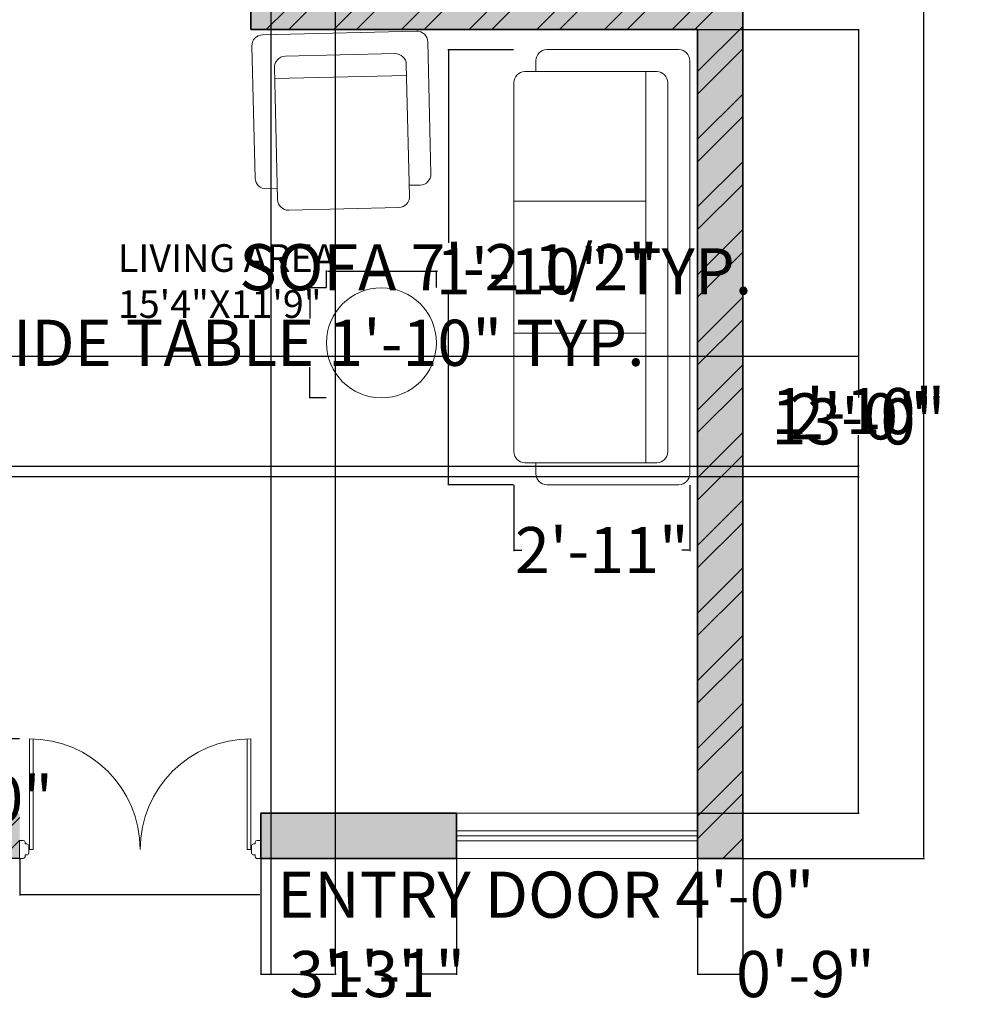
# Model space of a CAD drawing. Units: inches. Extents: x 1086 to 1540, y 3343 to 3848.
# Tile 2 of 8: x 1327 to 1515, y 3351 to 3547. Entities that reach past the tile are written whole.
import ezdxf

# ---------------------------------------------------------------- set-up
doc = ezdxf.new("R2010")
doc.units = ezdxf.units.IN
for name, color, linetype, lineweight in [('00 FURNITURE', 15, 'Continuous', 15), ('A-ANNO-DIMS', 2, 'Continuous', 13), ('A-AREA-IDEN', 7, 'Continuous', 18), ('A-DOOR', 4, 'Continuous', 20), ('A-WALL-PATT', 252, 'Continuous', 9), ('WALL', 7, 'Continuous', 35), ('WINDOW', 160, 'Continuous', 15)]:
    doc.layers.add(name, color=color, linetype=linetype, lineweight=lineweight)
doc.styles.get("Standard").update_dxf_attribs({"font": 'arial.ttf'})
doc.dimstyles.get("Standard").update_dxf_attribs({"dimtxt": 9.18, "dimasz": 0.18, "dimexe": 0.18, "dimexo": 0.0625, "dimgap": 0.09, "dimtad": 0, "dimtih": 1, "dimtoh": 1, "dimdec": 1, "dimzin": 0, "dimdsep": 46, "dimlunit": 3, "dimtxsty": 'Standard', "dimcen": 0.09, "dimadec": 0, "dimazin": 0, "dimtfac": 1, "dimtdec": 1, "dimtofl": 0, "dimtmove": 0, "dimatfit": 3, "dimfxl": 1, "dimtolj": 1, "dimtzin": 0, "dimarcsym": 0})

# ---------------------------------------------------------------- blocks, each defined once
blk = doc.blocks.new('PUJA')
at = {"layer": '00 FURNITURE'}
for p, q in [((-1941.8, -16091.75), (-1938.89, -16091.75)), ((-1941.8, -16092.33), (-1941.8, -16091.75)), ((-1938.89, -16091.75), (-1938.89, -16092.33)), ((-1940.35, -16093.35), (-1958.14, -16093.35)), ((-1940.35, -16093.93), (-1958.13, -16093.93)), ((-1941.22, -16092.62), (-1941.51, -16092.62)), ((-1940.35, -16093.35), (-1940.35, -16093.93)), ((-1939.18, -16092.62), (-1939.47, -16092.62)), ((-1940.35, -16128.93), (-1958.14, -16128.93)), ((-1940.35, -16128.35), (-1958.13, -16128.35)), ((-1940.35, -16128.93), (-1940.35, -16128.35)), ((-1941.8, -16129.96), (-1941.8, -16130.54)), ((-1941.8, -16130.54), (-1938.89, -16130.54)), ((-1941.22, -16129.66), (-1941.51, -16129.66)), ((-1939.18, -16129.66), (-1939.47, -16129.66)), ((-1938.89, -16130.54), (-1938.89, -16129.96))]:
    blk.add_line(p, q, dxfattribs=at)
for points in [[(-1939.47, -16092.62), (-1939.47, -16092.91, -0.414214), (-1939.76, -16093.21), (-1940.93, -16093.21, -0.414214), (-1941.22, -16092.91), (-1941.22, -16092.62)], [(-1939.47, -16129.66), (-1939.47, -16129.37, 0.414214), (-1939.76, -16129.08), (-1940.93, -16129.08, 0.414214), (-1941.22, -16129.37), (-1941.22, -16129.66)]]:
    blk.add_lwpolyline(points, format="xyb", dxfattribs=at)
for centre, radius, start, end in [((-1941.51, -16092.33), 0.292, 180, 270), ((-1939.18, -16092.33), 0.292, 270, 0), ((-1940.35, -16093.35), 17.79, 180, 270), ((-1940.35, -16128.93), 17.79, 90, 180), ((-1941.51, -16129.96), 0.292, 90, 180), ((-1939.18, -16129.96), 0.292, 0, 90)]:
    blk.add_arc(centre, radius, start, end, dxfattribs=at)
blk = doc.blocks.new('sofa 6')
for p, q in [((-1044.4, 890), (1044.4, 890)), ((-1100, 166.9), (-1100, 834.3)), ((1100, 834.3), (1100, 166.9)), ((-933.1, 778.7), (933.1, 778.7)), ((-988.8, 55.6), (-988.8, 723.1)), ((988.8, 723.1), (988.8, 55.6)), ((-988.8, 667.5), (988.8, 667.5)), ((-333.8, 667.5), (-333.8, 0)), ((333.7, 667.5), (333.7, 0)), ((-988.8, 111.2), (-1044.4, 111.2)), ((1044.4, 111.2), (988.8, 111.2)), ((933.1, 0), (-933.1, 0))]:
    blk.add_line(p, q)
for centre, start, end in [((-1044.4, 834.3), 90, 180), ((1044.4, 834.3), 0, 90), ((-933.1, 723.1), 90, 180), ((933.1, 723.1), 0, 90), ((-1044.4, 166.9), 180, 270), ((1044.4, 166.9), 270, 0), ((-933.1, 55.6), 180, 270), ((933.1, 55.6), 270, 0)]:
    blk.add_arc(centre, 55.6, start, end)
blk = doc.blocks.new('chair')
at = {"layer": '00 FURNITURE'}
for p, q in [((1375.85, 3529.75), (1402.12, 3529.75)), ((1373.66, 3525.37), (1373.66, 3527.56)), ((1404.31, 3527.56), (1404.31, 3496.9)), ((1371.47, 3525.37), (1397.74, 3525.37)), ((1395.55, 3525.37), (1395.55, 3499.09)), ((1369.28, 3501.28), (1369.28, 3523.18)), ((1399.93, 3523.18), (1399.93, 3501.28)), ((1397.74, 3499.09), (1371.47, 3499.09)), ((1373.66, 3496.9), (1373.66, 3499.09)), ((1402.12, 3494.71), (1375.85, 3494.71))]:
    blk.add_line(p, q, dxfattribs=at)
for centre, start, end in [((1375.85, 3527.56), 90, 180), ((1402.12, 3527.56), 0, 90), ((1371.47, 3523.18), 90, 180), ((1397.74, 3523.18), 0, 90), ((1371.47, 3501.28), 180, 270), ((1397.74, 3501.28), 270, 0), ((1375.85, 3496.9), 180, 270), ((1402.12, 3496.9), 270, 0)]:
    blk.add_arc(centre, 2.19, start, end, dxfattribs=at)
blk = doc.blocks.new('*D13')
at = {"layer": 'A-ANNO-DIMS', "color": 0, "lineweight": -2, "transparency": 16777216}
for p, q in [((1470.8, 3811.57), (1506.93, 3811.57)), ((1506.75, 3811.39), (1506.75, 3600.35)), ((1506.75, 3379.75), (1506.75, 3590.79)), ((1470.8, 3379.57), (1506.93, 3379.57))]:
    blk.add_line(p, q, dxfattribs=at)
at = {"layer": 'A-ANNO-DIMS', "color": 0, "transparency": 16777216}
for points in [[(1506.72, 3811.39), (1506.78, 3811.39), (1506.75, 3811.57)], [(1506.72, 3379.75), (1506.78, 3379.75), (1506.75, 3379.57)]]:
    blk.add_solid(points, dxfattribs=at)
at = {"layer": 'Defpoints', "color": 0, "transparency": 16777216}
for p in [(1470.74, 3811.57), (1470.74, 3379.57), (1506.75, 3379.57)]:
    blk.add_point(p, dxfattribs=at)
at = {"layer": 'A-ANNO-DIMS', "color": 0, "transparency": 16777216, "insert": (1506.75, 3595.57), "char_height": 9.18, "attachment_point": 5}
blk.add_mtext("\\A1;36'", dxfattribs=at)
blk = doc.blocks.new('WIN-GLAZING-48IN')
for p, q in [((48, 1), (0, 1)), ((48, 0), (0, 0)), ((48, -1), (0, -1))]:
    blk.add_line(p, q)
blk = doc.blocks.new('TABLE-ROUND-SIDE')
blk.add_circle((0, 0), 10.95)
blk = doc.blocks.new('*D29')
at = {"layer": 'A-ANNO-DIMS', "color": 0, "lineweight": -2, "transparency": 16777216}
for p, q in [((1387.77, 3493.16), (1384.37, 3493.16)), ((1384.55, 3492.98), (1384.55, 3487.04)), ((1384.55, 3471.44), (1384.55, 3477.37)), ((1387.77, 3471.26), (1384.37, 3471.26))]:
    blk.add_line(p, q, dxfattribs=at)
at = {"layer": 'A-ANNO-DIMS', "color": 0, "transparency": 16777216}
for points in [[(1384.52, 3492.98), (1384.58, 3492.98), (1384.55, 3493.16)], [(1384.52, 3471.44), (1384.58, 3471.44), (1384.55, 3471.26)]]:
    blk.add_solid(points, dxfattribs=at)
at = {"layer": 'Defpoints', "color": 0, "transparency": 16777216}
for p in [(1384.55, 3493.16), (1387.83, 3493.16), (1387.83, 3471.26)]:
    blk.add_point(p, dxfattribs=at)
at = {"layer": 'A-ANNO-DIMS', "color": 0, "transparency": 16777216, "insert": (1384.55, 3482.21), "char_height": 9.18, "attachment_point": 5}
blk.add_mtext('\\A1;SIDE TABLE 1\'-10" TYP.', dxfattribs=at)
blk = doc.blocks.new('*D30')
at = {"layer": 'A-ANNO-DIMS', "color": 0, "lineweight": -2, "transparency": 16777216}
for p, q in [((1387.83, 3493.22), (1387.83, 3496.62)), ((1388.01, 3496.44), (1409.55, 3496.44)), ((1409.73, 3493.22), (1409.73, 3496.62)), ((1409.73, 3496.44), (1409.91, 3496.44))]:
    blk.add_line(p, q, dxfattribs=at)
at = {"layer": 'A-ANNO-DIMS', "color": 0, "transparency": 16777216}
for points in [[(1388.01, 3496.47), (1388.01, 3496.41), (1387.83, 3496.44)], [(1409.55, 3496.47), (1409.55, 3496.41), (1409.73, 3496.44)]]:
    blk.add_solid(points, dxfattribs=at)
at = {"layer": 'Defpoints', "color": 0, "transparency": 16777216}
for p in [(1409.73, 3496.44), (1387.83, 3493.16), (1409.73, 3493.16)]:
    blk.add_point(p, dxfattribs=at)
at = {"layer": 'A-ANNO-DIMS', "color": 0, "transparency": 16777216, "insert": (1441.11, 3496.44), "char_height": 9.18, "attachment_point": 5}
blk.add_mtext('\\A1;1\'-10" TYP.', dxfattribs=at)
blk = doc.blocks.new('*D43')
at = {"layer": 'A-ANNO-DIMS', "color": 0, "lineweight": -2, "transparency": 16777216}
for p, q in [((1326.74, 3379.51), (1326.74, 3372.19)), ((1374.74, 3379.51), (1374.74, 3372.19)), ((1326.92, 3372.37), (1374.56, 3372.37)), ((1374.74, 3372.37), (1374.92, 3372.37))]:
    blk.add_line(p, q, dxfattribs=at)
at = {"layer": 'A-ANNO-DIMS', "color": 0, "transparency": 16777216}
for points in [[(1326.92, 3372.4), (1326.92, 3372.34), (1326.74, 3372.37)], [(1374.56, 3372.4), (1374.56, 3372.34), (1374.74, 3372.37)]]:
    blk.add_solid(points, dxfattribs=at)
at = {"layer": 'Defpoints', "color": 0, "transparency": 16777216}
for p in [(1326.74, 3379.57), (1374.74, 3379.57), (1374.74, 3372.37)]:
    blk.add_point(p, dxfattribs=at)
at = {"layer": 'A-ANNO-DIMS', "color": 0, "transparency": 16777216, "insert": (1431.5, 3372.37), "char_height": 9.18, "attachment_point": 5}
blk.add_mtext('\\A1;ENTRY DOOR 4\'-0"', dxfattribs=at)
blk = doc.blocks.new('*D44')
at = {"layer": 'A-ANNO-DIMS', "color": 0, "lineweight": -2, "transparency": 16777216}
for p, q in [((1326.68, 3403.39), (1319.36, 3403.39)), ((1319.54, 3403.21), (1319.54, 3396.26)), ((1319.54, 3379.75), (1319.54, 3386.7)), ((1326.68, 3379.57), (1319.36, 3379.57))]:
    blk.add_line(p, q, dxfattribs=at)
at = {"layer": 'A-ANNO-DIMS', "color": 0, "transparency": 16777216}
for points in [[(1319.51, 3403.21), (1319.57, 3403.21), (1319.54, 3403.39)], [(1319.51, 3379.75), (1319.57, 3379.75), (1319.54, 3379.57)]]:
    blk.add_solid(points, dxfattribs=at)
at = {"layer": 'Defpoints', "color": 0, "transparency": 16777216}
for p in [(1326.74, 3403.39), (1319.54, 3379.57), (1326.74, 3379.57)]:
    blk.add_point(p, dxfattribs=at)
at = {"layer": 'A-ANNO-DIMS', "color": 0, "transparency": 16777216, "insert": (1319.54, 3391.48), "char_height": 9.18, "attachment_point": 5}
blk.add_mtext('\\A1;2\'-0"', dxfattribs=at)
blk = doc.blocks.new('*D45')
at = {"layer": 'A-ANNO-DIMS', "color": 0, "lineweight": -2, "transparency": 16777216}
for p, q in [((1425.08, 3540.55), (1411.97, 3540.55)), ((1412.15, 3540.37), (1412.15, 3502.09)), ((1412.15, 3454.12), (1412.15, 3492.41)), ((1425.08, 3453.94), (1411.97, 3453.94))]:
    blk.add_line(p, q, dxfattribs=at)
at = {"layer": 'A-ANNO-DIMS', "color": 0, "transparency": 16777216}
for points in [[(1412.12, 3540.37), (1412.18, 3540.37), (1412.15, 3540.55)], [(1412.12, 3454.12), (1412.18, 3454.12), (1412.15, 3453.94)]]:
    blk.add_solid(points, dxfattribs=at)
at = {"layer": 'Defpoints', "color": 0, "transparency": 16777216}
for p in [(1425.14, 3540.55), (1412.15, 3453.94), (1425.14, 3453.94)]:
    blk.add_point(p, dxfattribs=at)
at = {"layer": 'A-ANNO-DIMS', "color": 0, "transparency": 16777216, "insert": (1412.15, 3497.25), "char_height": 9.18, "attachment_point": 5}
blk.add_mtext('\\A1;SOFA 7\'-2 1/2"', dxfattribs=at)
blk = doc.blocks.new('*D46')
at = {"layer": 'A-ANNO-DIMS', "color": 0, "lineweight": -2, "transparency": 16777216}
for p, q in [((1425.14, 3453.88), (1425.14, 3440.77)), ((1460.18, 3453.88), (1460.18, 3440.77)), ((1425.32, 3440.95), (1426.72, 3440.95)), ((1460, 3440.95), (1458.59, 3440.95))]:
    blk.add_line(p, q, dxfattribs=at)
at = {"layer": 'A-ANNO-DIMS', "color": 0, "transparency": 16777216}
for points in [[(1425.32, 3440.98), (1425.32, 3440.92), (1425.14, 3440.95)], [(1460, 3440.98), (1460, 3440.92), (1460.18, 3440.95)]]:
    blk.add_solid(points, dxfattribs=at)
at = {"layer": 'Defpoints', "color": 0, "transparency": 16777216}
for p in [(1425.14, 3453.94), (1460.18, 3453.94), (1460.18, 3440.95)]:
    blk.add_point(p, dxfattribs=at)
at = {"layer": 'A-ANNO-DIMS', "color": 0, "transparency": 16777216, "insert": (1442.66, 3440.95), "char_height": 9.18, "attachment_point": 5}
blk.add_mtext('\\A1;2\'-11"', dxfattribs=at)
blk = doc.blocks.new('*D49')
at = {"layer": 'A-ANNO-DIMS', "color": 0, "lineweight": -2, "transparency": 16777216}
for p, q in [((1374.74, 3379.51), (1374.74, 3356.39)), ((1413.74, 3379.51), (1413.74, 3356.39)), ((1374.92, 3356.57), (1381.95, 3356.57)), ((1413.56, 3356.57), (1406.53, 3356.57))]:
    blk.add_line(p, q, dxfattribs=at)
at = {"layer": 'A-ANNO-DIMS', "color": 0, "transparency": 16777216}
for points in [[(1374.92, 3356.6), (1374.92, 3356.54), (1374.74, 3356.57)], [(1413.56, 3356.6), (1413.56, 3356.54), (1413.74, 3356.57)]]:
    blk.add_solid(points, dxfattribs=at)
at = {"layer": 'Defpoints', "color": 0, "transparency": 16777216}
for p in [(1374.74, 3379.57), (1413.74, 3379.57), (1413.74, 3356.57)]:
    blk.add_point(p, dxfattribs=at)
at = {"layer": 'A-ANNO-DIMS', "color": 0, "transparency": 16777216, "insert": (1394.24, 3356.57), "char_height": 9.18, "attachment_point": 5}
blk.add_mtext('\\A1;3\'-3"', dxfattribs=at)
blk = doc.blocks.new('*D50')
at = {"layer": 'A-ANNO-DIMS', "color": 0, "lineweight": -2, "transparency": 16777216}
for p, q in [((1461.74, 3388.51), (1461.74, 3356.39)), ((1470.74, 3379.51), (1470.74, 3356.39)), ((1461.92, 3356.57), (1470.56, 3356.57)), ((1470.74, 3356.57), (1470.92, 3356.57))]:
    blk.add_line(p, q, dxfattribs=at)
at = {"layer": 'A-ANNO-DIMS', "color": 0, "transparency": 16777216}
for points in [[(1461.92, 3356.6), (1461.92, 3356.54), (1461.74, 3356.57)], [(1470.56, 3356.6), (1470.56, 3356.54), (1470.74, 3356.57)]]:
    blk.add_solid(points, dxfattribs=at)
at = {"layer": 'Defpoints', "color": 0, "transparency": 16777216}
for p in [(1461.74, 3388.57), (1470.74, 3379.57), (1470.74, 3356.57)]:
    blk.add_point(p, dxfattribs=at)
at = {"layer": 'A-ANNO-DIMS', "color": 0, "transparency": 16777216, "insert": (1483.21, 3356.57), "char_height": 9.18, "attachment_point": 5}
blk.add_mtext('\\A1;0\'-9"', dxfattribs=at)
blk = doc.blocks.new('*D57')
at = {"layer": 'A-ANNO-DIMS', "color": 0, "lineweight": -2, "transparency": 16777216}
for p, q in [((1318.8, 3479.57), (1493.92, 3479.57)), ((1493.74, 3479.39), (1493.74, 3472.35)), ((1493.74, 3455.75), (1493.74, 3462.79)), ((1318.8, 3455.57), (1493.92, 3455.57))]:
    blk.add_line(p, q, dxfattribs=at)
at = {"layer": 'A-ANNO-DIMS', "color": 0, "transparency": 16777216}
for points in [[(1493.71, 3479.39), (1493.77, 3479.39), (1493.74, 3479.57)], [(1493.71, 3455.75), (1493.77, 3455.75), (1493.74, 3455.57)]]:
    blk.add_solid(points, dxfattribs=at)
at = {"layer": 'Defpoints', "color": 0, "transparency": 16777216}
for p in [(1318.74, 3479.57), (1493.74, 3479.57), (1318.74, 3455.57)]:
    blk.add_point(p, dxfattribs=at)
at = {"layer": 'A-ANNO-DIMS', "color": 0, "transparency": 16777216, "insert": (1493.74, 3467.57), "char_height": 9.18, "attachment_point": 5}
blk.add_mtext('\\A1;2\'-0"', dxfattribs=at)
blk = doc.blocks.new('*D59')
at = {"layer": 'A-ANNO-DIMS', "color": 0, "lineweight": -2, "transparency": 16777216}
for p, q in [((1267.58, 3479.57), (1493.92, 3479.57)), ((1493.74, 3479.39), (1493.74, 3473.4)), ((1493.74, 3457.85), (1493.74, 3463.84)), ((1267.58, 3457.67), (1493.92, 3457.67))]:
    blk.add_line(p, q, dxfattribs=at)
at = {"layer": 'A-ANNO-DIMS', "color": 0, "transparency": 16777216}
for points in [[(1493.71, 3479.39), (1493.77, 3479.39), (1493.74, 3479.57)], [(1493.71, 3457.85), (1493.77, 3457.85), (1493.74, 3457.67)]]:
    blk.add_solid(points, dxfattribs=at)
at = {"layer": 'Defpoints', "color": 0, "transparency": 16777216}
for p in [(1267.52, 3479.57), (1493.74, 3479.57), (1267.52, 3457.67)]:
    blk.add_point(p, dxfattribs=at)
at = {"layer": 'A-ANNO-DIMS', "color": 0, "transparency": 16777216, "insert": (1493.74, 3468.62), "char_height": 9.18, "attachment_point": 5}
blk.add_mtext('\\A1;1\'-10"', dxfattribs=at)
blk = doc.blocks.new('*D66')
at = {"layer": 'A-ANNO-DIMS', "color": 0, "lineweight": -2, "transparency": 16777216}
for p, q in [((1376.74, 3548.51), (1376.74, 3356.39)), ((1389.55, 3548.8), (1389.55, 3356.39)), ((1376.92, 3356.57), (1389.37, 3356.57)), ((1389.55, 3356.57), (1389.73, 3356.57))]:
    blk.add_line(p, q, dxfattribs=at)
at = {"layer": 'A-ANNO-DIMS', "color": 0, "transparency": 16777216}
for points in [[(1376.92, 3356.6), (1376.92, 3356.54), (1376.74, 3356.57)], [(1389.37, 3356.6), (1389.37, 3356.54), (1389.55, 3356.57)]]:
    blk.add_solid(points, dxfattribs=at)
at = {"layer": 'Defpoints', "color": 0, "transparency": 16777216}
for p in [(1376.74, 3548.57), (1389.55, 3548.86), (1389.55, 3356.57)]:
    blk.add_point(p, dxfattribs=at)
at = {"layer": 'A-ANNO-DIMS', "color": 0, "transparency": 16777216, "insert": (1401.59, 3356.57), "char_height": 9.18, "attachment_point": 5}
blk.add_mtext('\\A1;1\'-1"', dxfattribs=at)
blk = doc.blocks.new('*D73')
at = {"layer": 'A-ANNO-DIMS', "color": 0, "lineweight": -2, "transparency": 16777216}
for p, q in [((1461.8, 3544.57), (1493.92, 3544.57)), ((1493.74, 3544.39), (1493.74, 3471.35)), ((1493.74, 3388.75), (1493.74, 3461.79)), ((1461.8, 3388.57), (1493.92, 3388.57))]:
    blk.add_line(p, q, dxfattribs=at)
at = {"layer": 'A-ANNO-DIMS', "color": 0, "transparency": 16777216}
for points in [[(1493.71, 3544.39), (1493.77, 3544.39), (1493.74, 3544.57)], [(1493.71, 3388.75), (1493.77, 3388.75), (1493.74, 3388.57)]]:
    blk.add_solid(points, dxfattribs=at)
at = {"layer": 'Defpoints', "color": 0, "transparency": 16777216}
for p in [(1461.74, 3544.57), (1493.74, 3544.57), (1461.74, 3388.57)]:
    blk.add_point(p, dxfattribs=at)
at = {"layer": 'A-ANNO-DIMS', "color": 0, "transparency": 16777216, "insert": (1493.74, 3466.57), "char_height": 9.18, "attachment_point": 5}
blk.add_mtext('\\A1;13\'-0"', dxfattribs=at)

msp = doc.modelspace()

# ---------------------------------------------------------------- hatches: boundary and pattern name
at = {"layer": 'A-WALL-PATT'}
h = msp.add_hatch(dxfattribs=at)
h.set_pattern_fill('ANSI32', color=256)
h.paths.add_polyline_path([(1234.55, 3811.57), (1234.55, 3811.57), (1194.74, 3811.57), (1194.74, 3622.57), (1203.74, 3622.57), (1203.74, 3634.57), (1218.33, 3634.57), (1218.33, 3638.57), (1203.74, 3638.57), (1203.74, 3802.57), (1234.55, 3802.57)])
h.paths.add_polyline_path([(1371.06, 3811.57), (1371.06, 3811.57), (1282.55, 3811.57), (1282.55, 3802.57), (1331.74, 3802.57), (1331.74, 3634.57), (1335.74, 3634.57), (1335.74, 3639.57), (1335.74, 3802.57), (1371.06, 3802.57)])
h.paths.add_polyline_path([(1470.74, 3811.57), (1419.06, 3811.57), (1419.06, 3802.57), (1461.74, 3802.57), (1461.74, 3638.57), (1461.74, 3548.57), (1425.74, 3548.57), (1425.74, 3582.21), (1421.74, 3582.21), (1421.74, 3548.57), (1376.74, 3548.57), (1376.74, 3602.57), (1373.71, 3602.57), (1372.74, 3602.57), (1372.74, 3544.57), (1461.74, 3544.57), (1461.74, 3379.57), (1470.74, 3379.57)])
h.paths.add_polyline_path([(1203.74, 3582.57), (1295.74, 3582.57), (1295.74, 3586.57), (1203.74, 3586.57), (1203.74, 3598.57), (1194.74, 3598.57), (1194.74, 3379.57), (1326.74, 3379.57), (1326.74, 3388.57), (1322.74, 3388.57), (1203.74, 3388.57), (1203.74, 3451.57), (1234.74, 3451.57), (1234.74, 3455.57), (1203.74, 3455.57), (1203.74, 3479.57), (1203.74, 3544.57), (1227.74, 3544.57), (1253.74, 3544.57), (1253.74, 3548.57), (1203.74, 3548.57)])
h.paths.add_polyline_path([(1461.74, 3638.57), (1371.74, 3638.57), (1371.74, 3634.57), (1372.74, 3634.57), (1372.74, 3632.57), (1376.74, 3632.57), (1376.74, 3634.57), (1421.74, 3634.57), (1421.74, 3606.21), (1425.74, 3606.21), (1425.74, 3634.57), (1461.74, 3634.57)])
h.paths.add_polyline_path([(1295.74, 3638.57), (1266.33, 3638.57), (1266.33, 3634.57), (1292.74, 3634.57), (1295.74, 3634.57)])
h.paths.add_polyline_path([(1322.74, 3548.57), (1318.74, 3548.57), (1318.74, 3455.57), (1282.74, 3455.57), (1282.74, 3451.57), (1318.74, 3451.57), (1318.74, 3420.07), (1322.74, 3420.07)], flags=17)
at = {"layer": 'A-WALL-PATT', "transparency": 33554559}
h = msp.add_hatch(color=256, dxfattribs=at)
h.dxf.hatch_style = 1
h.paths.add_polyline_path([(1234.55, 3811.57), (1234.55, 3811.57), (1194.74, 3811.57), (1194.74, 3622.57), (1203.74, 3622.57), (1203.74, 3634.57), (1218.33, 3634.57), (1218.33, 3638.57), (1203.74, 3638.57), (1203.74, 3802.57), (1234.55, 3802.57)])
h.paths.add_polyline_path([(1371.06, 3811.57), (1371.06, 3811.57), (1282.55, 3811.57), (1282.55, 3802.57), (1331.74, 3802.57), (1331.74, 3634.57), (1335.74, 3634.57), (1335.74, 3639.57), (1335.74, 3802.57), (1371.06, 3802.57)])
h.paths.add_polyline_path([(1470.74, 3811.57), (1419.06, 3811.57), (1419.06, 3802.57), (1461.74, 3802.57), (1461.74, 3638.57), (1461.74, 3548.57), (1425.74, 3548.57), (1425.74, 3582.21), (1421.74, 3582.21), (1421.74, 3548.57), (1376.74, 3548.57), (1376.74, 3602.57), (1372.74, 3602.57), (1372.74, 3544.57), (1461.74, 3544.57), (1461.74, 3379.57), (1470.74, 3379.57)])
h.paths.add_polyline_path([(1203.74, 3544.57), (1227.74, 3544.57), (1253.74, 3544.57), (1253.74, 3548.57), (1203.74, 3548.57), (1203.74, 3582.57), (1295.74, 3582.57), (1295.74, 3586.57), (1203.74, 3586.57), (1203.74, 3598.57), (1194.74, 3598.57), (1194.74, 3379.57), (1326.74, 3379.57), (1326.74, 3388.57), (1322.74, 3388.57), (1203.74, 3388.57), (1203.74, 3451.57), (1234.74, 3451.57), (1234.74, 3455.57), (1203.74, 3455.57)])
h.paths.add_polyline_path([(1413.74, 3388.57), (1413.74, 3388.57), (1374.74, 3388.57), (1374.74, 3383.18), (1374.74, 3383.18), (1374.74, 3379.57), (1413.74, 3379.57)], flags=17)
h.paths.add_polyline_path([(1322.74, 3548.57), (1318.74, 3548.57), (1318.74, 3455.57), (1282.74, 3455.57), (1282.74, 3451.57), (1318.74, 3451.57), (1318.74, 3420.07), (1322.74, 3420.07)], flags=17)
h.paths.add_polyline_path([(1295.74, 3638.57), (1266.33, 3638.57), (1266.33, 3634.57), (1292.74, 3634.57), (1295.74, 3634.57)])
h.paths.add_polyline_path([(1461.74, 3638.57), (1371.74, 3638.57), (1371.74, 3634.57), (1372.74, 3634.57), (1372.74, 3632.57), (1376.74, 3632.57), (1376.74, 3634.57), (1421.74, 3634.57), (1421.74, 3606.21), (1425.74, 3606.21), (1425.74, 3634.57), (1461.74, 3634.57)])

# ---------------------------------------------------------------- linework, layer by layer
at = {"layer": 'WALL'}
for p, q in [((1470.74, 3811.57), (1470.74, 3379.57)), ((1372.74, 3602.57), (1372.74, 3544.57)), ((1372.74, 3544.57), (1461.74, 3544.57)), ((1461.74, 3544.57), (1461.74, 3379.57)), ((1413.74, 3388.57), (1374.74, 3388.57)), ((1374.74, 3379.57), (1374.74, 3388.57)), ((1413.74, 3388.57), (1413.74, 3379.57)), ((1413.74, 3379.57), (1374.74, 3379.57)), ((1470.74, 3379.57), (1461.74, 3379.57))]:
    msp.add_line(p, q, dxfattribs=at)
at = {"layer": 'WINDOW'}
for p, q in [((1461.74, 3388.57), (1413.74, 3388.57)), ((1413.74, 3379.57), (1461.74, 3379.57))]:
    msp.add_line(p, q, dxfattribs=at)

# ---------------------------------------------------------------- block references
at = {"layer": '00 FURNITURE', "rotation": 91.40028059934971}
msp.add_blockref('chair', (4935.93, 2225.81), dxfattribs=at)
at = {"layer": '00 FURNITURE', "xscale": 0.0393700787401575, "yscale": 0.0393700787401575, "zscale": 0.0393700787401575, "rotation": 270}
msp.add_blockref('sofa 6', (1425.14, 3497.25), dxfattribs=at)
at = {"layer": '00 FURNITURE'}
msp.add_blockref('TABLE-ROUND-SIDE', (1398.78, 3482.21), dxfattribs=at)
at = {"layer": 'A-DOOR', "xscale": 1.237379162154587, "yscale": 1.237379162154587, "zscale": 1.237379162154587, "rotation": 270.0000000034012}
msp.add_blockref('PUJA', (21286.33, 980.43), dxfattribs=at)
at = {"layer": 'WINDOW'}
msp.add_blockref('WIN-GLAZING-48IN', (1413.74, 3384.07), dxfattribs=at)

# ---------------------------------------------------------------- texts
at = {"layer": 'A-AREA-IDEN', "insert": (1346.29, 3501.83), "char_height": 8, "attachment_point": 1}
msp.add_mtext_dynamic_manual_height_columns('{\\H0.6875x;LIVING AREA\\P15\'4"X11\'9"\\H1.1818x; }  ', width=58.9878, gutter_width=0, heights=[37.04], dxfattribs=at)

# ---------------------------------------------------------------- dimensions: what is measured, and where the dimension line sits
at = {"layer": 'A-ANNO-DIMS'}
for base, p1, p2, angle, override, picture, middle in [((1506.75, 3379.57), (1470.74, 3811.57), (1470.74, 3379.57), 90, {"dimclrd": 0, "dimclre": 0, "dimclrt": 0}, '*D13', (1506.75, 3595.57)), ((1493.74, 3544.57), (1461.74, 3388.57), (1461.74, 3544.57), 90, {"dimdec": 1, "dimlfac": 1, "dimrnd": 0, "dimzin": 1, "dimdsep": 46, "dimlunit": 4, "dimfrac": 2}, '*D73', (1493.74, 3466.57)), ((1493.74, 3479.57), (1267.52, 3457.67), (1267.52, 3479.57), 90, {"dimdec": 1, "dimlfac": 1, "dimrnd": 0, "dimzin": 1, "dimdsep": 46, "dimlunit": 4, "dimfrac": 2}, '*D59', (1493.74, 3468.62)), ((1493.74, 3479.57), (1318.74, 3455.57), (1318.74, 3479.57), 90, {"dimdec": 1, "dimlfac": 1, "dimrnd": 0, "dimzin": 1, "dimdsep": 46, "dimlunit": 4, "dimfrac": 2}, '*D57', (1493.74, 3467.57)), ((1319.54, 3379.57), (1326.74, 3403.39), (1326.74, 3379.57), 270, {"dimdec": 1, "dimlfac": 1, "dimrnd": 0, "dimzin": 1, "dimdsep": 46, "dimlunit": 4, "dimfrac": 2}, '*D44', (1319.54, 3391.48))]:
    dim = msp.add_linear_dim(base=base, p1=p1, p2=p2, angle=angle, dimstyle='Standard', override=override, dxfattribs=at)
    dim.commit()
    dim.dimension.update_dxf_attribs({"geometry": picture, "text_midpoint": middle})
for base, p1, p2, picture, middle in [((1389.55, 3356.57), (1376.74, 3548.57), (1389.55, 3548.86), '*D66', (1401.59, 3356.57)), ((1460.18, 3440.95), (1425.14, 3453.94), (1460.18, 3453.94), '*D46', (1442.66, 3440.95)), ((1470.74, 3356.57), (1461.74, 3388.57), (1470.74, 3379.57), '*D50', (1483.21, 3356.57)), ((1413.74, 3356.57), (1374.74, 3379.57), (1413.74, 3379.57), '*D49', (1394.24, 3356.57))]:
    dim = msp.add_linear_dim(base=base, p1=p1, p2=p2, dimstyle='Standard', override={"dimdec": 1, "dimlfac": 1, "dimrnd": 0, "dimzin": 1, "dimdsep": 46, "dimlunit": 4, "dimfrac": 2}, dxfattribs=at)
    dim.commit()
    dim.dimension.update_dxf_attribs({"geometry": picture, "text_midpoint": middle})
for base, p1, p2, angle, text, picture, middle in [((1412.15, 3453.94), (1425.14, 3540.55), (1425.14, 3453.94), 270, 'SOFA <>', '*D45', (1412.15, 3497.25)), ((1384.55, 3493.16), (1387.83, 3471.26), (1387.83, 3493.16), 90, 'SIDE TABLE <> TYP.', '*D29', (1384.55, 3482.21)), ((1374.74, 3372.37), (1326.74, 3379.57), (1374.74, 3379.57), 0, 'ENTRY DOOR <>', '*D43', (1431.5, 3372.37))]:
    dim = msp.add_linear_dim(base=base, p1=p1, p2=p2, angle=angle, text=text, dimstyle='Standard', override={"dimdec": 1, "dimlfac": 1, "dimrnd": 0, "dimzin": 1, "dimdsep": 46, "dimlunit": 4, "dimfrac": 2}, dxfattribs=at)
    dim.commit()
    dim.dimension.update_dxf_attribs({"geometry": picture, "text_midpoint": middle})
dim = msp.add_linear_dim(base=(1409.73, 3496.44), p1=(1387.83, 3493.16), p2=(1409.73, 3493.16), text='<> TYP.', dimstyle='Standard', override={"dimdec": 1, "dimlfac": 1, "dimrnd": 0, "dimzin": 1, "dimdsep": 46, "dimlunit": 4, "dimfrac": 2}, dxfattribs=at)
dim.commit()
dim.dimension.update_dxf_attribs({"geometry": '*D30', "text_midpoint": (1441.11, 3496.44)})

doc.saveas('drawing.dxf')
